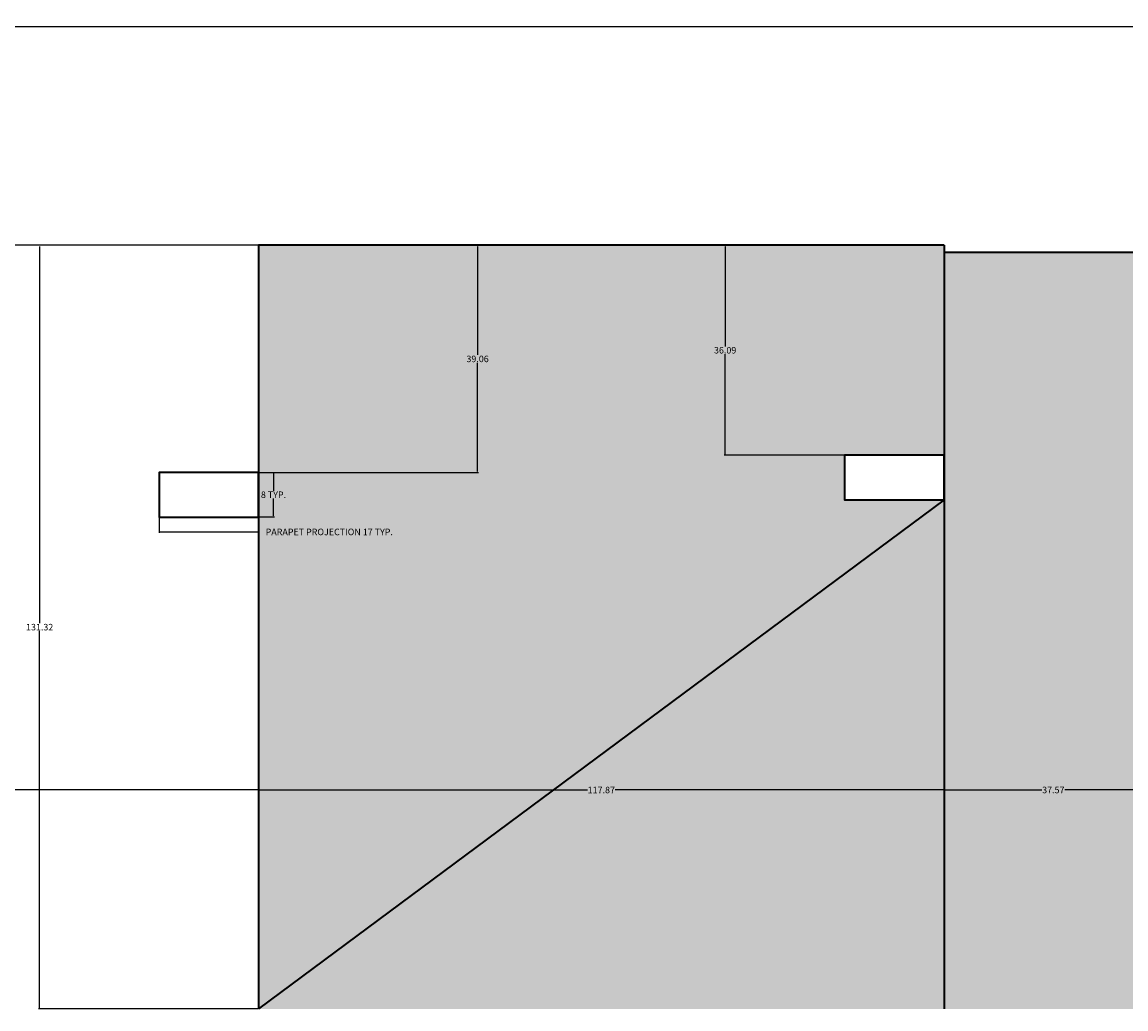
# Model space of a CAD drawing. Units: inches. Extents: x 8 to 634, y 41 to 867.
# Tile 17 of 21: x 104 to 293, y 698 to 867. Entities that reach past the tile are written whole.
import ezdxf

# ---------------------------------------------------------------- set-up
doc = ezdxf.new("R2010")
doc.units = ezdxf.units.IN
doc.header["$MEASUREMENT"] = 0
for name, color, linetype, lineweight in [('A-ANNO-DIMS', 2, 'Continuous', 18), ('A-ELEV-PATT', 252, 'Continuous', 9), ('A-ROOF', 7, 'Continuous', 35), ('A-ROOF-PATT', 8, 'Continuous', 9)]:
    doc.layers.add(name, color=color, linetype=linetype, lineweight=lineweight)
doc.styles.get("Standard").update_dxf_attribs({"font": 'arial.ttf'})
doc.dimstyles.get("Standard").update_dxf_attribs({"dimtxt": 1.125, "dimasz": 0.18, "dimexe": 0.18, "dimexo": 0.0625, "dimgap": 0.09, "dimtad": 0, "dimtih": 1, "dimtoh": 1, "dimdec": 4, "dimzin": 0, "dimdsep": 46, "dimlunit": 4, "dimtxsty": 'Standard', "dimcen": 0.09, "dimadec": 0, "dimazin": 0, "dimtfac": 1, "dimtdec": 4, "dimtofl": 0, "dimtmove": 0, "dimatfit": 3, "dimfxl": 1, "dimtolj": 1, "dimtzin": 0, "dimarcsym": 0})

# ---------------------------------------------------------------- blocks, each defined once
blk = doc.blocks.new('PARAPET-PROJECTION')
blk.add_lwpolyline([(17.11, 7.66), (0, 7.66), (0, 0), (17.11, 0)], close=True)
blk = doc.blocks.new('*D17')
at = {"layer": 'A-ANNO-DIMS', "color": 0, "lineweight": -2, "transparency": 16777216}
for p, q in [((127.24, 782.19), (127.24, 779.51)), ((144.36, 782.19), (144.36, 779.51)), ((127.42, 779.69), (144.18, 779.69)), ((144.36, 779.69), (144.54, 779.69))]:
    blk.add_line(p, q, dxfattribs=at)
at = {"layer": 'A-ANNO-DIMS', "color": 0, "transparency": 16777216}
for points in [[(127.42, 779.72), (127.42, 779.66), (127.24, 779.69)], [(144.18, 779.72), (144.18, 779.66), (144.36, 779.69)]]:
    blk.add_solid(points, dxfattribs=at)
at = {"layer": 'Defpoints', "color": 0, "transparency": 16777216}
for p in [(127.24, 782.26), (144.36, 782.26), (144.36, 779.69)]:
    blk.add_point(p, dxfattribs=at)
at = {"layer": 'A-ANNO-DIMS', "color": 0, "transparency": 16777216, "insert": (156.51, 779.69), "char_height": 1.125, "attachment_point": 5}
blk.add_mtext('\\A1;PARAPET PROJECTION 17 TYP.', dxfattribs=at)
blk = doc.blocks.new('*D18')
at = {"layer": 'A-ANNO-DIMS', "color": 0, "lineweight": -2, "transparency": 16777216}
for p, q in [((144.42, 789.92), (147.1, 789.92)), ((146.92, 789.74), (146.92, 786.75)), ((146.92, 782.44), (146.92, 785.42)), ((144.42, 782.26), (147.1, 782.26))]:
    blk.add_line(p, q, dxfattribs=at)
at = {"layer": 'A-ANNO-DIMS', "color": 0, "transparency": 16777216}
for points in [[(146.89, 789.74), (146.95, 789.74), (146.92, 789.92)], [(146.89, 782.44), (146.95, 782.44), (146.92, 782.26)]]:
    blk.add_solid(points, dxfattribs=at)
at = {"layer": 'Defpoints', "color": 0, "transparency": 16777216}
for p in [(144.36, 789.92), (146.92, 789.92), (144.36, 782.26)]:
    blk.add_point(p, dxfattribs=at)
at = {"layer": 'A-ANNO-DIMS', "color": 0, "transparency": 16777216, "insert": (146.92, 786.09), "char_height": 1.125, "attachment_point": 5}
blk.add_mtext('\\A1;8 TYP.', dxfattribs=at)
blk = doc.blocks.new('*D19')
at = {"layer": 'A-ANNO-DIMS', "color": 0, "lineweight": -2, "transparency": 16777216}
for p, q in [((47.34, 697.73), (47.34, 866.81)), ((47.52, 866.63), (319.51, 866.63)), ((594.17, 866.63), (322.18, 866.63)), ((594.35, 827.83), (594.35, 866.81))]:
    blk.add_line(p, q, dxfattribs=at)
at = {"layer": 'A-ANNO-DIMS', "color": 0, "transparency": 16777216}
for points in [[(47.52, 866.66), (47.52, 866.6), (47.34, 866.63)], [(594.17, 866.66), (594.17, 866.6), (594.35, 866.63)]]:
    blk.add_solid(points, dxfattribs=at)
at = {"layer": 'Defpoints', "color": 0, "transparency": 16777216}
for p in [(594.35, 866.63), (594.35, 827.77), (47.34, 697.67)]:
    blk.add_point(p, dxfattribs=at)
at = {"layer": 'A-ANNO-DIMS', "color": 0, "transparency": 16777216, "insert": (320.85, 866.63), "char_height": 1.125, "attachment_point": 5}
blk.add_mtext('\\A1;547', dxfattribs=at)
blk = doc.blocks.new('*D20')
at = {"layer": 'A-ANNO-DIMS', "color": 0, "lineweight": -2, "transparency": 16777216}
for p, q in [((144.29, 828.98), (9.51, 828.98)), ((9.69, 828.8), (9.69, 454.93)), ((9.69, 79.74), (9.69, 453.6)), ((47.28, 79.56), (9.51, 79.56))]:
    blk.add_line(p, q, dxfattribs=at)
at = {"layer": 'A-ANNO-DIMS', "color": 0, "transparency": 16777216}
for points in [[(9.66, 828.8), (9.72, 828.8), (9.69, 828.98)], [(9.66, 79.74), (9.72, 79.74), (9.69, 79.56)]]:
    blk.add_solid(points, dxfattribs=at)
at = {"layer": 'Defpoints', "color": 0, "transparency": 16777216}
for p in [(9.69, 828.98), (144.36, 828.98), (47.34, 79.56)]:
    blk.add_point(p, dxfattribs=at)
at = {"layer": 'A-ANNO-DIMS', "color": 0, "transparency": 16777216, "insert": (9.69, 454.27), "char_height": 1.125, "attachment_point": 5}
blk.add_mtext('\\A1;749.4', dxfattribs=at)
blk = doc.blocks.new('*D21')
at = {"layer": 'A-ANNO-DIMS', "color": 0, "lineweight": -2, "transparency": 16777216}
for p, q in [((144.29, 828.98), (106.53, 828.98)), ((106.71, 828.8), (106.71, 763.99)), ((106.71, 697.85), (106.71, 762.66)), ((144.29, 697.67), (106.53, 697.67))]:
    blk.add_line(p, q, dxfattribs=at)
at = {"layer": 'A-ANNO-DIMS', "color": 0, "transparency": 16777216}
for points in [[(106.68, 828.8), (106.74, 828.8), (106.71, 828.98)], [(106.68, 697.85), (106.74, 697.85), (106.71, 697.67)]]:
    blk.add_solid(points, dxfattribs=at)
at = {"layer": 'Defpoints', "color": 0, "transparency": 16777216}
for p in [(106.71, 828.98), (144.36, 828.98), (144.36, 697.67)]:
    blk.add_point(p, dxfattribs=at)
at = {"layer": 'A-ANNO-DIMS', "color": 0, "transparency": 16777216, "insert": (106.71, 763.32), "char_height": 1.125, "attachment_point": 5}
blk.add_mtext('\\A1;131.32', dxfattribs=at)
blk = doc.blocks.new('*D22')
at = {"layer": 'A-ANNO-DIMS', "color": 0, "lineweight": -2, "transparency": 16777216}
for p, q in [((47.34, 697.73), (47.34, 735.5)), ((47.52, 735.32), (93.87, 735.32)), ((144.18, 735.32), (97.83, 735.32)), ((144.36, 697.73), (144.36, 735.5))]:
    blk.add_line(p, q, dxfattribs=at)
at = {"layer": 'A-ANNO-DIMS', "color": 0, "transparency": 16777216}
for points in [[(47.52, 735.35), (47.52, 735.29), (47.34, 735.32)], [(144.18, 735.35), (144.18, 735.29), (144.36, 735.32)]]:
    blk.add_solid(points, dxfattribs=at)
at = {"layer": 'Defpoints', "color": 0, "transparency": 16777216}
for p in [(144.36, 735.32), (47.34, 697.67), (144.36, 697.67)]:
    blk.add_point(p, dxfattribs=at)
at = {"layer": 'A-ANNO-DIMS', "color": 0, "transparency": 16777216, "insert": (95.85, 735.32), "char_height": 1.125, "attachment_point": 5}
blk.add_mtext('\\A1;97.02', dxfattribs=at)
blk = doc.blocks.new('*D23')
at = {"layer": 'A-ANNO-DIMS', "color": 0, "lineweight": -2, "transparency": 16777216}
for p, q in [((144.36, 697.73), (144.36, 735.5)), ((144.54, 735.32), (200.92, 735.32)), ((262.05, 735.32), (205.66, 735.32)), ((262.23, 697.73), (262.23, 735.5))]:
    blk.add_line(p, q, dxfattribs=at)
at = {"layer": 'A-ANNO-DIMS', "color": 0, "transparency": 16777216}
for points in [[(144.54, 735.35), (144.54, 735.29), (144.36, 735.32)], [(262.05, 735.35), (262.05, 735.29), (262.23, 735.32)]]:
    blk.add_solid(points, dxfattribs=at)
at = {"layer": 'Defpoints', "color": 0, "transparency": 16777216}
for p in [(262.23, 735.32), (144.36, 697.67), (262.23, 697.67)]:
    blk.add_point(p, dxfattribs=at)
at = {"layer": 'A-ANNO-DIMS', "color": 0, "transparency": 16777216, "insert": (203.29, 735.32), "char_height": 1.125, "attachment_point": 5}
blk.add_mtext('\\A1;117.87', dxfattribs=at)
blk = doc.blocks.new('*D24')
at = {"layer": 'A-ANNO-DIMS', "color": 0, "lineweight": -2, "transparency": 16777216}
for p, q in [((262.23, 697.73), (262.23, 735.5)), ((262.41, 735.32), (279.02, 735.32)), ((299.62, 735.32), (283, 735.32)), ((299.8, 697.73), (299.8, 735.5))]:
    blk.add_line(p, q, dxfattribs=at)
at = {"layer": 'A-ANNO-DIMS', "color": 0, "transparency": 16777216}
for points in [[(262.41, 735.35), (262.41, 735.29), (262.23, 735.32)], [(299.62, 735.35), (299.62, 735.29), (299.8, 735.32)]]:
    blk.add_solid(points, dxfattribs=at)
at = {"layer": 'Defpoints', "color": 0, "transparency": 16777216}
for p in [(299.8, 735.32), (262.23, 697.67), (299.8, 697.67)]:
    blk.add_point(p, dxfattribs=at)
at = {"layer": 'A-ANNO-DIMS', "color": 0, "transparency": 16777216, "insert": (281.01, 735.32), "char_height": 1.125, "attachment_point": 5}
blk.add_mtext('\\A1;37.57', dxfattribs=at)
blk = doc.blocks.new('*D26')
at = {"layer": 'A-ANNO-DIMS', "color": 0, "lineweight": -2, "transparency": 16777216}
for p, q in [((144.42, 828.98), (182.19, 828.98)), ((182.01, 828.8), (182.01, 810.12)), ((182.01, 790.1), (182.01, 808.79)), ((144.42, 789.92), (182.19, 789.92))]:
    blk.add_line(p, q, dxfattribs=at)
at = {"layer": 'A-ANNO-DIMS', "color": 0, "transparency": 16777216}
for points in [[(181.98, 828.8), (182.04, 828.8), (182.01, 828.98)], [(181.98, 790.1), (182.04, 790.1), (182.01, 789.92)]]:
    blk.add_solid(points, dxfattribs=at)
at = {"layer": 'Defpoints', "color": 0, "transparency": 16777216}
for p in [(144.36, 828.98), (144.36, 789.92), (182.01, 789.92)]:
    blk.add_point(p, dxfattribs=at)
at = {"layer": 'A-ANNO-DIMS', "color": 0, "transparency": 16777216, "insert": (182.01, 809.45), "char_height": 1.125, "attachment_point": 5}
blk.add_mtext('\\A1;39.06', dxfattribs=at)
blk = doc.blocks.new('*D27')
at = {"layer": 'A-ANNO-DIMS', "color": 0, "lineweight": -2, "transparency": 16777216}
for p, q in [((262.16, 828.98), (224.4, 828.98)), ((224.58, 828.8), (224.58, 811.6)), ((224.58, 793.07), (224.58, 810.27)), ((262.16, 792.89), (224.4, 792.89))]:
    blk.add_line(p, q, dxfattribs=at)
at = {"layer": 'A-ANNO-DIMS', "color": 0, "transparency": 16777216}
for points in [[(224.55, 828.8), (224.61, 828.8), (224.58, 828.98)], [(224.55, 793.07), (224.61, 793.07), (224.58, 792.89)]]:
    blk.add_solid(points, dxfattribs=at)
at = {"layer": 'Defpoints', "color": 0, "transparency": 16777216}
for p in [(224.58, 828.98), (262.23, 828.98), (262.23, 792.89)]:
    blk.add_point(p, dxfattribs=at)
at = {"layer": 'A-ANNO-DIMS', "color": 0, "transparency": 16777216, "insert": (224.58, 810.94), "char_height": 1.125, "attachment_point": 5}
blk.add_mtext('\\A1;36.09', dxfattribs=at)

msp = doc.modelspace()

# ---------------------------------------------------------------- hatches: boundary and pattern name
at = {"layer": 'A-ELEV-PATT', "transparency": 33554687}
h = msp.add_hatch(color=256, dxfattribs=at)
h.dxf.hatch_style = 1
h.paths.add_polyline_path([(262.2266, 785.231), (144.3564, 697.6655), (262.2266, 697.6655)])
at = {"layer": 'A-ROOF-PATT', "transparency": 33554687}
h = msp.add_hatch(dxfattribs=at)
h.set_pattern_fill('AR-CONC', color=256, scale=2.2, angle=135)
h.paths.add_polyline_path([(262.2266, 828.9821), (144.3564, 828.9821), (144.3564, 697.6655), (262.2266, 785.231), (245.114, 785.231), (245.114, 792.8938), (262.2266, 792.8938)])
h.paths.add_polyline_path([(594.3501, 827.7671), (262.2266, 827.7671), (262.2266, 792.8938), (262.2266, 697.6655), (299.7961, 697.6655), (299.7961, 776.8929), (556.7072, 776.8929), (556.7072, 774.3342), (556.7072, 697.6655), (594.3501, 697.6655)])

# ---------------------------------------------------------------- linework, layer by layer
at = {"layer": 'A-ROOF'}
for p, q in [((262.2266, 828.9821), (144.3564, 828.9821)), ((144.3564, 828.9821), (144.3564, 697.6655)), ((262.2266, 828.9821), (262.2266, 697.6655)), ((594.3501, 827.7671), (262.2266, 827.7671)), ((262.2266, 785.231), (144.3564, 697.6655))]:
    msp.add_line(p, q, dxfattribs=at)

# ---------------------------------------------------------------- block references
for p in [(245.1142, 785.2311), (127.244, 782.257)]:
    msp.add_blockref('PARAPET-PROJECTION', p, dxfattribs=at)

# ---------------------------------------------------------------- dimensions: what is measured, and where the dimension line sits
at = {"layer": 'A-ANNO-DIMS'}
for base, p1, p2, override, picture, middle in [((594.3501, 866.6321), (47.3401, 697.6655), (594.3501, 827.7671), {"dimdec": 0, "dimlfac": 1, "dimrnd": 0, "dimzin": 0, "dimdsep": 46, "dimlunit": 2}, '*D19', (320.8451, 866.6321)), ((144.3564, 735.3155), (47.3401, 697.6655), (144.3564, 697.6655), {"dimdec": 2, "dimlfac": 1, "dimrnd": 0, "dimzin": 0, "dimdsep": 46, "dimlunit": 2}, '*D22', (95.8482, 735.3155)), ((262.2266, 735.3155), (144.3564, 697.6655), (262.2266, 697.6655), {"dimdec": 2, "dimlfac": 1, "dimrnd": 0, "dimzin": 0, "dimdsep": 46, "dimlunit": 2}, '*D23', (203.2915, 735.3155)), ((299.7961, 735.3155), (262.2266, 697.6655), (299.7961, 697.6655), {"dimdec": 2, "dimlfac": 1, "dimrnd": 0, "dimzin": 0, "dimdsep": 46, "dimlunit": 2}, '*D24', (281.0113, 735.3155))]:
    dim = msp.add_linear_dim(base=base, p1=p1, p2=p2, dimstyle='Standard', override=override, dxfattribs=at)
    dim.commit()
    dim.dimension.update_dxf_attribs({"geometry": picture, "text_midpoint": middle})
for base, p1, p2, angle, override, picture, middle in [((9.6901, 828.9821), (47.3401, 79.5555), (144.3564, 828.9821), 90, {"dimdec": 1, "dimlfac": 1, "dimrnd": 0, "dimzin": 0, "dimdsep": 46, "dimlunit": 2}, '*D20', (9.6901, 454.2688)), ((106.7064, 828.9821), (144.3564, 697.6655), (144.3564, 828.9821), 90, {"dimdec": 2, "dimlfac": 1, "dimrnd": 0, "dimzin": 0, "dimdsep": 46, "dimlunit": 2}, '*D21', (106.7064, 763.3238)), ((182.0064, 789.9198), (144.3564, 828.9821), (144.3564, 789.9198), 270, {"dimdec": 2, "dimlfac": 1, "dimrnd": 0, "dimzin": 0, "dimdsep": 46, "dimlunit": 2}, '*D26', (182.0064, 809.4509)), ((224.5766, 828.9821), (262.2266, 792.8938), (262.2266, 828.9821), 90, {"dimdec": 2, "dimlfac": 1, "dimrnd": 0, "dimzin": 0, "dimdsep": 46, "dimlunit": 2}, '*D27', (224.5766, 810.9379))]:
    dim = msp.add_linear_dim(base=base, p1=p1, p2=p2, angle=angle, dimstyle='Standard', override=override, dxfattribs=at)
    dim.commit()
    dim.dimension.update_dxf_attribs({"geometry": picture, "text_midpoint": middle})
dim = msp.add_linear_dim(base=(146.9233, 789.9198), p1=(144.3564, 782.2569), p2=(144.3564, 789.9198), angle=90, text='<> TYP.', dimstyle='Standard', override={"dimdec": 0, "dimlfac": 1, "dimrnd": 0, "dimzin": 0, "dimdsep": 46, "dimlunit": 2}, dxfattribs=at)
dim.commit()
dim.dimension.update_dxf_attribs({"geometry": '*D18', "text_midpoint": (146.9233, 786.0883)})
dim = msp.add_linear_dim(base=(144.3564, 779.69), p1=(127.2438, 782.2569), p2=(144.3564, 782.2569), text='PARAPET PROJECTION <> TYP.', dimstyle='Standard', override={"dimdec": 0, "dimlfac": 1, "dimrnd": 0, "dimzin": 0, "dimdsep": 46, "dimlunit": 2}, dxfattribs=at)
dim.commit()
dim.dimension.update_dxf_attribs({"geometry": '*D17', "text_midpoint": (156.5057, 779.69)})

doc.saveas('drawing.dxf')
